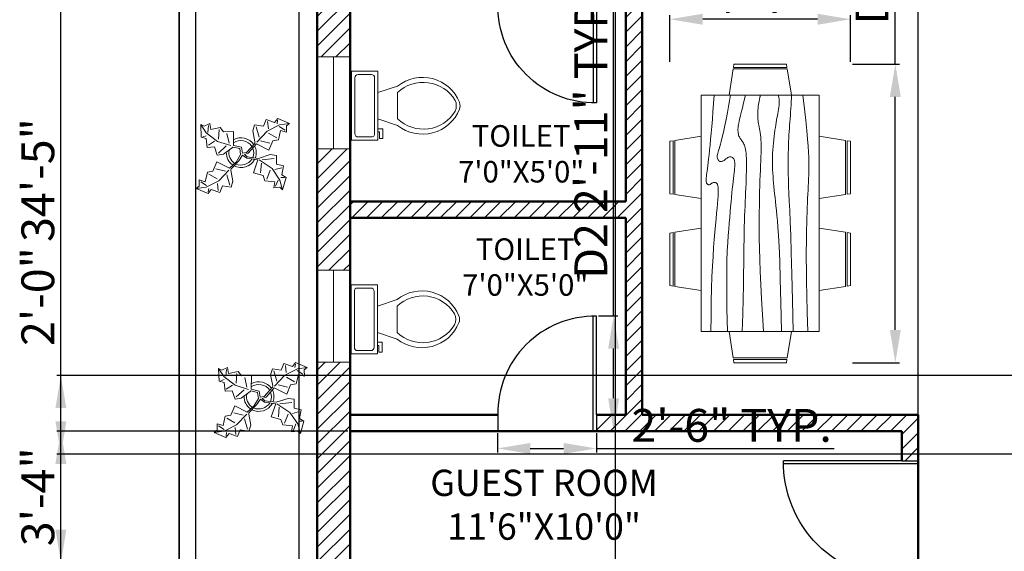
# Model space of a CAD drawing. Units: inches. Extents: x 2206 to 2843, y 1750 to 2489.
# Tile 5 of 8: x 2206 to 2506, y 2075 to 2237. Entities that reach past the tile are written whole.
import ezdxf

# ---------------------------------------------------------------- set-up
doc = ezdxf.new("R2010")
doc.units = ezdxf.units.IN
for name, color, linetype, lineweight in [('A-ANNO-DIMS', 2, 'Continuous', 18), ('A-AREA-IDEN', 7, 'Continuous', 18), ('A-DOOR', 3, 'Continuous', 25), ('A-FLOR-FIXT', 9, 'Continuous', 18), ('A-FURN', 21, 'Continuous', 18), ('A-GLAZ', 4, 'Continuous', 18), ('A-WALL', 7, 'Continuous', 50), ('A-WALL-PATT', 252, 'Continuous', 13), ('C-PROP', 7, 'Continuous', 35), ('L-PLNT', 92, 'Continuous', 18), ('L-SITE-WALL', 8, 'Continuous', 25)]:
    doc.layers.add(name, color=color, linetype=linetype, lineweight=lineweight)
doc.styles.get("Standard").update_dxf_attribs({"font": 'arial.ttf'})
doc.dimstyles.new('ISO-25', dxfattribs={"dimtxt": 10, "dimasz": 10, "dimexe": 1.25, "dimexo": 0.625, "dimtad": 1, "dimdec": 1, "dimlunit": 3, "dimtxsty": 'Standard', "dimcen": 2.5, "dimadec": 0, "dimazin": 0, "dimtfac": 1, "dimtdec": 1, "dimtmove": 0, "dimatfit": 3, "dimfxl": 1, "dimarcsym": 0})

# ---------------------------------------------------------------- blocks, each defined once
blk = doc.blocks.new('Dining Set - 36 x 72 in.')
for p, q in [((-22, 27.5), (-22.1562, 26.50042)), ((-22, 27.5), (-6, 27.5)), ((-5.8437, 26.49966), (-6, 27.5)), ((6, 27.5), (5.8438, 26.50042)), ((6, 27.5), (22, 27.5)), ((22.1563, 26.49966), (22, 27.5)), ((-22.2343, 26.00059), (-23.4847, 17.99762)), ((-22.2304, 26), (-5.7608, 26)), ((-5.8416, 26.5), (-22.1534, 26.5)), ((-4.5152, 17.99762), (-5.7655, 25.99926)), ((5.7657, 26.00059), (4.5153, 17.99762)), ((5.7696, 26), (22.2392, 26)), ((22.1584, 26.5), (5.8466, 26.5)), ((23.4848, 17.99762), (22.2345, 25.99926)), ((36, 18), (-36, 18)), ((-36, 18), (-36, -18)), ((36, -18), (36, 18)), ((-44.0006, 8.23428), (-35.9976, 9.48474)), ((44.0006, 8.23428), (35.9976, 9.48474)), ((-45.5, 8), (-44.5004, 8.15617)), ((-45.5, 8), (-45.5, -8)), ((-44.5, -8.15843), (-44.5, 8.15338)), ((-44, 8.23041), (-44, -8.23915)), ((44, 8.23041), (44, -8.23915)), ((44.5, -8.15843), (44.5, 8.15338)), ((45.5, 8), (44.5005, 8.15617)), ((45.5, 8), (45.5, -8)), ((-44.4997, -8.15631), (-45.5, -8)), ((-35.9976, -9.48476), (-43.9993, -8.2345)), ((35.9976, -9.48476), (43.9993, -8.2345)), ((44.4997, -8.15631), (45.5, -8)), ((-36, -18), (36, -18)), ((-22.2343, -26.0006), (-23.4847, -17.99762)), ((-4.5152, -17.99762), (-5.7655, -25.99928)), ((5.7657, -26.0006), (4.5153, -17.99762)), ((23.4848, -17.99762), (22.2345, -25.99928)), ((-22.2304, -26), (-5.7608, -26)), ((-22, -27.5), (-22.1562, -26.50044)), ((-5.8416, -26.5), (-22.1534, -26.5)), ((-5.8437, -26.49967), (-6, -27.5)), ((5.7696, -26), (22.2392, -26)), ((6, -27.5), (5.8438, -26.50044)), ((22.1584, -26.5), (5.8466, -26.5)), ((22.1563, -26.49967), (22, -27.5)), ((-22, -27.5), (-6, -27.5)), ((6, -27.5), (22, -27.5))]:
    blk.add_line(p, q)
for points in [[(-36, 15), (-31.1772, 14.97754), (-26.8079, 14.91406), (-22.8538, 14.81543), (-19.276, 14.6875), (-16.0362, 14.53613), (-13.0957, 14.36718), (-10.4159, 14.18652), (-7.9583, 14), (-5.6904, 13.81315), (-3.6035, 13.63021), (-1.6954, 13.45508), (0.0365, 13.29166), (1.5945, 13.14388), (2.9811, 13.01562), (4.1988, 12.9108), (5.25, 12.83333), (6.1393, 12.78613), (6.8802, 12.76823), (7.4883, 12.77767), (7.9792, 12.8125), (8.3685, 12.87077), (8.6719, 12.95052), (8.9049, 13.0498), (9.0833, 13.16666), (9.2205, 13.29899), (9.3216, 13.44401), (9.3895, 13.59879), (9.4271, 13.76041), (9.4373, 13.92594), (9.4232, 14.09245), (9.3875, 14.257), (9.3333, 14.41666), (9.2638, 14.56917), (9.1836, 14.71484), (9.0975, 14.85465), (9.0104, 14.98958), (8.9272, 15.1206), (8.8529, 15.2487), (8.7922, 15.37483), (8.75, 15.5), (8.7305, 15.62467), (8.7344, 15.74739), (8.7617, 15.86621), (8.8125, 15.97916), (8.8867, 16.08431), (8.9844, 16.17968), (9.1055, 16.26334), (9.25, 16.33333), (9.4189, 16.38802), (9.6172, 16.42708), (9.8506, 16.45052), (10.125, 16.45833), (10.4463, 16.45052), (10.8203, 16.42708), (11.2529, 16.38802), (11.75, 16.33333), (12.3184, 16.26318), (12.9694, 16.17838), (13.7151, 16.07991), (14.5677, 15.96875), (15.5395, 15.84586), (16.6426, 15.71224), (17.8893, 15.56884), (19.2917, 15.41666), (20.859, 15.25667), (22.5879, 15.08984), (24.4721, 14.91715), (26.5052, 14.73958), (28.6809, 14.5581), (30.9929, 14.3737), (33.4347, 14.18733), (36, 14)], [(-36, 10), (-28.9766, 10.14274), (-23.1725, 10.20442), (-18.4241, 10.19775), (-14.5677, 10.13541), (-11.4399, 10.03011), (-8.877, 9.89453), (-6.7154, 9.74137), (-4.7917, 9.58333), (-2.9698, 9.43082), (-1.2246, 9.28515), (0.4415, 9.14534), (2.026, 9.01041), (3.5266, 8.87939), (4.9408, 8.7513), (6.266, 8.62516), (7.5, 8.5), (8.6411, 8.37549), (9.6914, 8.2539), (10.6538, 8.13818), (11.5312, 8.03125), (12.3267, 7.93603), (13.043, 7.85547), (13.6831, 7.79248), (14.25, 7.75), (14.7471, 7.7303), (15.1797, 7.73307), (15.5537, 7.75732), (15.875, 7.80208), (16.1494, 7.86637), (16.3828, 7.94922), (16.5811, 8.04964), (16.75, 8.16666), (16.8944, 8.29915), (17.0143, 8.44531), (17.1089, 8.60319), (17.1771, 8.77083), (17.218, 8.94629), (17.2305, 9.1276), (17.2137, 9.31282), (17.1667, 9.5), (17.0895, 9.6875), (16.987, 9.875), (16.8649, 10.0625), (16.7292, 10.25), (16.5856, 10.4375), (16.4401, 10.625), (16.2985, 10.8125), (16.1667, 11), (16.05, 11.18733), (15.9518, 11.3737), (15.8752, 11.5581), (15.8229, 11.73958), (15.798, 11.91715), (15.8034, 12.08984), (15.842, 12.25667), (15.9167, 12.41666), (16.0295, 12.56836), (16.1784, 12.70833), (16.3605, 12.83268), (16.5729, 12.9375), (16.8127, 13.01888), (17.0768, 13.07291), (17.3625, 13.0957), (17.6667, 13.08333), (17.9894, 13.03312), (18.3418, 12.94726), (18.7382, 12.82918), (19.1927, 12.68229), (19.7195, 12.51001), (20.3327, 12.31575), (21.0465, 12.10294), (21.875, 11.875), (22.8357, 11.63354), (23.959, 11.37304), (25.2786, 11.08618), (26.8282, 10.76562), (28.6414, 10.40405), (30.752, 9.99414), (33.1936, 9.52856), (36, 9)], [(-36, 5.5), (-30.7157, 5.3348), (-26.069, 5.20963), (-21.9946, 5.11767), (-18.4271, 5.05208), (-15.3009, 5.00602), (-12.5508, 4.97265), (-10.1112, 4.94515), (-7.9167, 4.91666), (-5.909, 4.88167), (-4.0586, 4.83984), (-2.3429, 4.79215), (-0.7396, 4.73958), (0.7739, 4.6831), (2.22, 4.6237), (3.6213, 4.56233), (5, 4.5), (6.373, 4.43782), (7.7344, 4.3776), (9.0723, 4.32129), (10.375, 4.27083), (11.6309, 4.22819), (12.8281, 4.19531), (13.9551, 4.17415), (15, 4.16666), (15.954, 4.17448), (16.819, 4.19791), (17.6001, 4.23698), (18.3021, 4.29166), (18.9299, 4.36198), (19.4883, 4.44791), (19.9823, 4.54948), (20.4167, 4.66666), (20.7969, 4.79899), (21.1302, 4.94401), (21.4245, 5.09879), (21.6875, 5.26041), (21.9271, 5.42594), (22.1511, 5.59245), (22.3672, 5.757), (22.5834, 5.91666), (22.8065, 6.06868), (23.0404, 6.21093), (23.2879, 6.34147), (23.5521, 6.45833), (23.8358, 6.55957), (24.142, 6.64323), (24.4735, 6.70735), (24.8334, 6.75), (25.2235, 6.76969), (25.642, 6.76692), (26.0858, 6.74267), (26.5521, 6.69791), (27.0379, 6.63362), (27.5404, 6.55078), (28.0565, 6.45036), (28.5834, 6.33333), (29.1242, 6.19987), (29.7071, 6.04687), (30.3661, 5.87044), (31.1354, 5.66666), (32.0493, 5.43164), (33.142, 5.16146), (34.4475, 4.85221), (36, 4.5)], [(-36, -1), (-30.7915, -0.6591), (-26.0195, -0.38216), (-21.6519, -0.16284), (-17.6563, 0.00521), (-14.0005, 0.12833), (-10.6523, 0.21289), (-7.5796, 0.26522), (-4.75, 0.29166), (-2.134, 0.29793), (0.2878, 0.28711), (2.5317, 0.26163), (4.6146, 0.22396), (6.5529, 0.17651), (8.3633, 0.12174), (10.0623, 0.06209), (11.6667, 0), (13.1899, -0.06201), (14.6341, -0.1211), (15.9982, -0.17432), (17.2813, -0.21875), (18.4823, -0.25147), (19.6003, -0.26953), (20.6343, -0.27002), (21.5834, -0.25), (22.4481, -0.20768), (23.2357, -0.14584), (23.9549, -0.06836), (24.6146, 0.02083), (25.2235, 0.11784), (25.7904, 0.21875), (26.3241, 0.31966), (26.8334, 0.41666), (27.3265, 0.50618), (27.8099, 0.58593), (28.2894, 0.65397), (28.7709, 0.70833), (29.2601, 0.74707), (29.763, 0.76823), (30.2855, 0.76985), (30.8334, 0.75), (31.4088, 0.70784), (31.9994, 0.64713), (32.589, 0.57275), (33.1615, 0.48958), (33.7008, 0.4025), (34.1908, 0.3164), (34.6153, 0.23616), (34.9584, 0.16666), (35.2099, 0.11165), (35.3848, 0.07031), (35.504, 0.04069), (35.5886, 0.02083), (35.6594, 0.00879), (35.7377, 0.0026), (35.8442, 0.00032), (36, 0)], [(-36, -6.5), (-27.1843, -6.31267), (-20.084, -6.1263), (-14.469, -5.9419), (-10.1094, -5.76042), (-6.7752, -5.58285), (-4.2363, -5.41016), (-2.2629, -5.24333), (-0.625, -5.08334), (0.8708, -4.93099), (2.2715, -4.78646), (3.5872, -4.64974), (4.8281, -4.52084), (6.0046, -4.39974), (7.127, -4.28646), (8.2053, -4.18099), (9.25, -4.08334), (10.2705, -3.99382), (11.2734, -3.91407), (12.2647, -3.84603), (13.25, -3.79167), (14.2354, -3.75293), (15.2266, -3.73177), (16.2295, -3.73015), (17.25, -3.75), (18.2912, -3.79248), (19.3451, -3.85547), (20.4009, -3.93604), (21.4479, -4.03125), (22.4754, -4.13819), (23.4727, -4.25391), (24.4289, -4.37549), (25.3334, -4.5), (26.1785, -4.62492), (26.9694, -4.74935), (27.7145, -4.87281), (28.4219, -4.99479), (29.1, -5.11483), (29.7572, -5.23242), (30.4016, -5.34709), (31.0417, -5.45834), (31.6837, -5.56437), (32.3262, -5.65821), (32.9658, -5.73153), (33.599, -5.77604), (34.2224, -5.78345), (34.8327, -5.74545), (35.4264, -5.65373), (36, -5.5)], [(-36, -10), (-26.4022, -9.81299), (-18.4675, -9.62891), (-11.9839, -9.45069), (-6.7396, -9.28125), (-2.5226, -9.12354), (0.8789, -8.98047), (3.6769, -8.85498), (6.0833, -8.75), (8.2767, -8.66765), (10.3021, -8.60677), (12.1712, -8.56543), (13.8958, -8.54167), (15.4876, -8.53353), (16.9583, -8.53907), (18.3197, -8.55632), (19.5834, -8.58334), (20.7616, -8.61841), (21.8685, -8.66081), (22.9188, -8.71004), (23.9271, -8.76563), (24.9081, -8.82707), (25.8763, -8.89388), (26.8465, -8.96558), (27.8334, -9.04167), (28.8474, -9.12118), (29.8828, -9.20117), (30.93, -9.27824), (31.9792, -9.34896), (33.0205, -9.40991), (34.0443, -9.45768), (35.0407, -9.48885), (36, -9.5)], [(-36, -14.5), (-30.0881, -14.33513), (-25.0332, -14.21224), (-20.7312, -14.12647), (-17.0781, -14.07292), (-13.97, -14.04671), (-11.3027, -14.04297), (-8.9724, -14.05681), (-6.875, -14.08334), (-4.9224, -14.11833), (-3.0905, -14.16016), (-1.3709, -14.20785), (0.2448, -14.26042), (1.7647, -14.3169), (3.1973, -14.3763), (4.5507, -14.43767), (5.8333, -14.5), (7.0554, -14.5621), (8.235, -14.62175), (9.3922, -14.67652), (10.5469, -14.72396), (11.7192, -14.76164), (12.929, -14.78711), (14.1965, -14.79794), (15.5417, -14.79167), (16.9933, -14.76424), (18.6152, -14.70508), (20.4804, -14.60197), (22.6615, -14.44271), (25.2312, -14.21509), (28.2624, -13.9069), (31.8277, -13.50594), (36, -13)]]:
    blk.add_lwpolyline(points)
blk = doc.blocks.new('Toilet - top')
for p, q in [((9.5, -6), (9.5, -2)), ((-10, -8.5), (-8, -8.5)), ((-10, -9.5), (-10, -8.5)), ((-8, -8.5), (-8, -8)), ((-7, -8), (-7, -9.5)), ((-4, -8), (-6, -14)), ((4, -8), (6, -14)), ((-7, -9.5), (-10, -9.5)), ((4, -14), (-4, -14))]:
    blk.add_line(p, q)
blk.add_lwpolyline([(10.5, -8), (10.5, 0), (-10.5, 0), (-10.5, -8)], close=True)
for points in [[(-9.5, -2), (-9.5, -6)], [(8.5, -1), (-8.5, -1)], [(-8.5, -7), (8.5, -7)]]:
    blk.add_lwpolyline(points)
for centre, radius, start, end in [((-8.62, -1.88), 0.884, 81.8699, 188.1301), ((8.62, -1.88), 0.884, 351.8699, 98.1301), ((-8.62, -6.12), 0.884, 171.8699, 278.1301), ((8.62, -6.12), 0.884, 261.8699, 8.1301), ((3.52, -21.58), 12.17, 141.4691, 247.9714), ((4.2, -21.82), 11.33, 136.3677, 238.9468), ((-3.52, -21.58), 12.17, 292.0284, 38.5307), ((-4.2, -21.82), 11.33, 301.053, 43.6321), ((0, -27.88), 4, 245.7318, 294.2682), ((0, -29), 4, 254.8605, 285.1395)]:
    blk.add_arc(centre, radius, start, end)
blk = doc.blocks.new('Plant - Rubber or Philodendron')
for p, q in [((-14.8639, 10.7964), (-12.6195, 11.8975)), ((-12.6195, 11.8975), (-12.1909, 9.4345)), ((8.8871, 10.7908), (9.9809, 13.4933)), ((9.9809, 13.4933), (13.3837, 12.301)), ((10.5828, 12.6946), (10.8893, 9.7953)), ((13.3837, 12.301), (14.68, 13.9039)), ((14.5816, 13.2037), (14.3848, 11.8033)), ((14.68, 13.9039), (19.3848, 11.8146)), ((-16.2005, 11.4774), (-13.9899, 8.1064)), ((-16.2005, 11.4774), (-14.8639, 10.7964)), ((-16.0159, 6.3329), (-16.2005, 11.4774)), ((-13.9899, 8.1064), (-9.5434, 4.7185)), ((-13.3174, 8.325), (-13.0735, 11.0065)), ((-12.1909, 9.4345), (-8.3829, 10.3)), ((-8.8369, 9.409), (-9.0894, 5.6095)), ((-8.3829, 10.3), (-7.0549, 8.501)), ((-7.0549, 8.501), (-3.0284, 8.6941)), ((-3.0284, 8.6941), (-3.0709, 3.1041)), ((4.6914, 8.8812), (5.3859, 11.2828)), ((4.6914, 8.8812), (5.5014, 4.4831)), ((5.3859, 11.2828), (8.8871, 10.7908)), ((5.9878, 10.4842), (7.1971, 6.3869)), ((10.3916, 8.7942), (6.2847, 4.4028)), ((15.3859, 11.3055), (10.3916, 8.7942)), ((14.2977, 6.1031), (10.9934, 7.9956)), ((15.7909, 9.1065), (14.8995, 5.3044)), ((15.2875, 10.6053), (17.5907, 9.2105)), ((19.3848, 11.8146), (15.3859, 11.3055)), ((18.1925, 8.4119), (15.7909, 9.1065)), ((19.3848, 11.8146), (18.1868, 10.9119)), ((18.1868, 10.9119), (18.1925, 8.4119)), ((-14.0069, 5.8704), (-16.0159, 6.3329)), ((-15.3434, 6.5514), (-13.9984, 6.9884)), ((-13.5868, 2.2894), (-14.0069, 5.8704)), ((-13.1329, 3.1804), (-10.6614, 4.727)), ((-9.5434, 4.7185), (-4.1917, 2.9888)), ((-4.8529, 4.012), (-5.7184, 7.82)), ((5.4346, 3.9146), (5.5014, 4.4831)), ((7.7005, 4.8881), (11.5025, 3.9967)), ((12.7005, 4.8994), (11.1089, 1.1958)), ((14.8995, 5.3044), (12.7005, 4.8994)), ((-10.6784, 2.491), (-13.5868, 2.2894)), ((-9.5858, -0.8715), (-10.6784, 2.491)), ((-9.1318, 0.0195), (-5.9793, 2.9025)), ((-7.1228, -0.443), (-3.5248, 2.2131)), ((-3.5248, 2.2131), (-3.3011, 2.4355)), ((-3.3011, 2.4355), (-0.5306, 1.7947)), ((-3.0709, 3.1041), (0.0797, 2.3163)), ((-0.5306, 1.7947), (-0.2255, -0.5527)), ((-0.5306, 1.7947), (-0.5306, 1.7947)), ((0.0797, 2.3163), (0.4866, -0.031)), ((0.4866, -0.031), (2.1141, 0.2298)), ((2.1141, 0.2298), (5.4346, 3.9146)), ((6.1032, 3.6844), (2.8262, -0.031)), ((11.1089, 1.1958), (6.1032, 3.6844)), ((-11.3237, -7.2629), (-9.7321, -3.5593)), ((-9.7321, -3.5593), (-4.7264, -6.0479)), ((-7.1228, -0.443), (-9.5858, -0.8715)), ((-2.019, -3.6148), (-4.7264, -6.0479)), ((-4.0579, -6.2781), (-0.9375, -3.1608)), ((-2.019, -3.6148), (-0.2255, -0.5527)), ((-0.9375, -3.1608), (0.5883, -0.8135)), ((0.5883, -0.8135), (2.2447, -2.0916)), ((2.8262, -0.031), (1.3003, -0.5527)), ((1.3003, -0.5527), (2.4193, -1.4655)), ((2.2447, -2.0916), (6.7108, -2.6626)), ((2.4193, -1.4655), (6.895, -2.1175)), ((4.943, -7.9659), (6.7108, -2.6626)), ((11.6605, -0.5413), (6.895, -2.1175)), ((12.3677, -6.1981), (7.219, -2.6772)), ((8.3544, -2.7453), (13.1973, -2.1704)), ((11.6605, -0.5413), (14.1354, -0.8948)), ((14.1354, -0.8948), (14.1354, -4.4304)), ((-14.4141, -11.4699), (-13.5228, -7.6679)), ((-13.5228, -7.6679), (-11.3237, -7.2629)), ((-6.3237, -7.2516), (-10.1257, -6.3602)), ((-9.0148, -11.1577), (-4.9047, -6.8122)), ((-4.1246, -6.8466), (-4.0579, -6.2781)), ((-3.3146, -11.2447), (-4.1246, -6.8466)), ((8.125, -4.0768), (7.7715, -7.9659)), ((10.2463, -10.4408), (11.6605, -6.9053)), ((15.5496, -10.7943), (12.3677, -6.1981)), ((16.2567, -5.8446), (13.4283, -6.5517)), ((14.1354, -4.4304), (16.9638, -5.1375)), ((16.9638, -5.1375), (16.2567, -8.673)), ((-16.8157, -10.7754), (-14.4141, -11.4699)), ((-16.8101, -13.2754), (-16.8157, -10.7754)), ((-13.9107, -12.9688), (-16.2139, -11.574)), ((-14.0091, -13.669), (-9.0148, -11.1577)), ((-12.921, -8.4665), (-9.6166, -10.359)), ((-4.611, -12.8477), (-5.8203, -8.7504)), ((-3.3146, -11.2447), (-4.0092, -13.6463)), ((8.8321, -9.0266), (4.943, -7.9659)), ((9.5392, -11.1479), (8.8321, -9.0266)), ((13.4283, -11.5015), (9.5392, -11.1479)), ((13.0748, -13.9763), (13.4283, -11.5015)), ((14.8425, -10.7943), (13.7819, -13.2692)), ((16.6103, -14.6834), (15.5496, -10.7943)), ((17.3174, -9.7337), (15.9032, -9.7337)), ((16.2567, -8.673), (18.0245, -9.7337)), ((18.0245, -9.7337), (16.6103, -14.6834)), ((-18.008, -14.1781), (-16.8101, -13.2754)), ((-18.008, -14.1781), (-14.0091, -13.669)), ((-13.3032, -16.2674), (-18.008, -14.1781)), ((-12.0069, -14.6645), (-13.3032, -16.2674)), ((-13.2048, -15.5672), (-13.008, -14.1668)), ((-8.6042, -15.8568), (-12.0069, -14.6645)), ((-9.206, -15.0581), (-9.5126, -12.1588)), ((-7.5103, -13.1543), (-8.6042, -15.8568)), ((-4.0092, -13.6463), (-7.5103, -13.1543)), ((15.5496, -13.6228), (13.0748, -13.9763)), ((16.6103, -14.6834), (15.5496, -13.6228))]:
    blk.add_line(p, q)
for centre, radius, start, end in [((0, 0), 6.1275, 34.37569, 120.1028), ((-0.0601, -0.2075), 5.2461, 33.82192, 124.9414), ((0.0308, 0.1664), 6, 178.6147, 235.1169), ((0.0308, 0.1664), 5, 168.1647, 238.6725), ((-0.2664, 0.1682), 5.2775, 338.4094, 20.03007), ((-0.098, 0.1364), 6.1288, 341.2017, 26.09184), ((-0.0234, 0.3825), 6.1492, 242.5812, 331.2714), ((-0.1102, 0.4886), 5.2883, 247.3711, 327.472)]:
    blk.add_arc(centre, radius, start, end)
blk = doc.blocks.new('WIN-28IN')
for p, q in [((10, 28), (0, 28)), ((5, 28), (5, 0)), ((10, 0), (0, 0))]:
    blk.add_line(p, q)
blk = doc.blocks.new('DOOR-SWING-36IN')
for p, q in [((0, 5), (0, 41)), ((1, 0), (1, 41)), ((0, 5), (0, 0)), ((36, 5), (36, 0))]:
    blk.add_line(p, q)
blk.add_arc((0.5, 5.5), 35.5, 359.1931, 90.8069)
blk = doc.blocks.new('DOOR-SWING-30IN')
for p, q in [((29, 0), (29, 35)), ((30, 5), (30, 35))]:
    blk.add_line(p, q)
blk.add_arc((29.5, 5.5), 29.5, 89.029, 180.971)
blk = doc.blocks.new('*D43')
at = {"layer": 'A-ANNO-DIMS', "color": 0, "lineweight": -2, "transparency": 16777216}
for p, q in [((2386.85, 2147.03), (2386.85, 2248.25)), ((2382.2, 2147.03), (2388.1, 2147.03)), ((2386.85, 2121.9), (2386.85, 2137.03)), ((2382.2, 2111.9), (2388.1, 2111.9))]:
    blk.add_line(p, q, dxfattribs=at)
at = {"layer": 'A-ANNO-DIMS', "color": 0, "transparency": 16777216}
for points in [[(2385.18, 2137.03), (2388.52, 2137.03), (2386.85, 2147.03)], [(2385.18, 2121.9), (2388.52, 2121.9), (2386.85, 2111.9)]]:
    blk.add_solid(points, dxfattribs=at)
at = {"layer": 'Defpoints', "color": 0, "transparency": 16777216}
for p in [(2381.58, 2147.03), (2386.85, 2147.03), (2381.58, 2111.9)]:
    blk.add_point(p, dxfattribs=at)
at = {"layer": 'A-ANNO-DIMS', "color": 0, "transparency": 16777216, "insert": (2381.2, 2202.64), "char_height": 10, "attachment_point": 5, "rotation": 90}
blk.add_mtext('D2 2\'-11" TYP.', dxfattribs=at)
blk = doc.blocks.new('*D44')
at = {"layer": 'A-ANNO-DIMS', "color": 0, "lineweight": -2, "transparency": 16777216}
for p, q in [((2351.44, 2111.27), (2351.44, 2105.38)), ((2381.58, 2111.27), (2381.58, 2105.38)), ((2361.44, 2106.63), (2371.58, 2106.63)), ((2381.58, 2106.63), (2453.96, 2106.63))]:
    blk.add_line(p, q, dxfattribs=at)
at = {"layer": 'A-ANNO-DIMS', "color": 0, "transparency": 16777216}
for points in [[(2361.44, 2108.3), (2361.44, 2104.96), (2351.44, 2106.63)], [(2371.58, 2108.3), (2371.58, 2104.96), (2381.58, 2106.63)]]:
    blk.add_solid(points, dxfattribs=at)
at = {"layer": 'Defpoints', "color": 0, "transparency": 16777216}
for p in [(2351.44, 2111.9), (2381.58, 2111.9), (2381.58, 2106.63)]:
    blk.add_point(p, dxfattribs=at)
at = {"layer": 'A-ANNO-DIMS', "color": 0, "transparency": 16777216, "insert": (2422.77, 2112.36), "char_height": 10, "attachment_point": 5}
blk.add_mtext('2\'-6" TYP.', dxfattribs=at)
blk = doc.blocks.new('*D47')
at = {"layer": 'A-ANNO-DIMS', "color": 0, "lineweight": -2, "transparency": 16777216}
for p, q in [((2472.62, 2223.74), (2472.62, 2344.9)), ((2459.59, 2223.74), (2473.87, 2223.74)), ((2472.62, 2142.74), (2472.62, 2213.74)), ((2459.59, 2132.74), (2473.87, 2132.74))]:
    blk.add_line(p, q, dxfattribs=at)
at = {"layer": 'A-ANNO-DIMS', "color": 0, "transparency": 16777216}
for points in [[(2470.95, 2213.74), (2474.28, 2213.74), (2472.62, 2223.74)], [(2470.95, 2142.74), (2474.28, 2142.74), (2472.62, 2132.74)]]:
    blk.add_solid(points, dxfattribs=at)
at = {"layer": 'Defpoints', "color": 0, "transparency": 16777216}
for p in [(2458.97, 2223.74), (2472.62, 2223.74), (2458.97, 2132.74)]:
    blk.add_point(p, dxfattribs=at)
at = {"layer": 'A-ANNO-DIMS', "color": 0, "transparency": 16777216, "insert": (2466.82, 2289.32), "char_height": 10, "attachment_point": 5, "rotation": 90}
blk.add_mtext('DINING SET 7\'-7"', dxfattribs=at)
blk = doc.blocks.new('*D48')
at = {"layer": 'A-ANNO-DIMS', "color": 0, "lineweight": -2, "transparency": 16777216}
for p, q in [((2403.97, 2224.37), (2403.97, 2238.64)), ((2448.97, 2237.39), (2413.97, 2237.39)), ((2458.97, 2224.37), (2458.97, 2238.64))]:
    blk.add_line(p, q, dxfattribs=at)
at = {"layer": 'A-ANNO-DIMS', "color": 0, "transparency": 16777216}
for points in [[(2413.97, 2239.06), (2413.97, 2235.73), (2403.97, 2237.39)], [(2448.97, 2239.06), (2448.97, 2235.73), (2458.97, 2237.39)]]:
    blk.add_solid(points, dxfattribs=at)
at = {"layer": 'Defpoints', "color": 0, "transparency": 16777216}
for p in [(2403.97, 2237.39), (2403.97, 2223.74), (2458.97, 2223.74)]:
    blk.add_point(p, dxfattribs=at)
at = {"layer": 'A-ANNO-DIMS', "color": 0, "transparency": 16777216, "insert": (2431.47, 2243.02), "char_height": 10, "attachment_point": 5}
blk.add_mtext('4\'-7"', dxfattribs=at)
blk = doc.blocks.new('*D58')
at = {"layer": 'A-ANNO-DIMS', "color": 0, "lineweight": -2, "transparency": 16777216}
for p, q in [((2295.95, 2394.9), (2217.28, 2394.9)), ((2218.53, 1991.9), (2218.53, 2384.9)), ((2295.95, 1981.9), (2217.28, 1981.9))]:
    blk.add_line(p, q, dxfattribs=at)
at = {"layer": 'A-ANNO-DIMS', "color": 0, "transparency": 16777216}
for points in [[(2216.86, 2384.9), (2220.2, 2384.9), (2218.53, 2394.9)], [(2216.86, 1991.9), (2220.2, 1991.9), (2218.53, 1981.9)]]:
    blk.add_solid(points, dxfattribs=at)
at = {"layer": 'Defpoints', "color": 0, "transparency": 16777216}
for p in [(2218.53, 2394.9), (2296.58, 2394.9), (2296.58, 1981.9)]:
    blk.add_point(p, dxfattribs=at)
at = {"layer": 'A-ANNO-DIMS', "color": 0, "transparency": 16777216, "insert": (2212.8, 2188.4), "char_height": 10, "attachment_point": 5, "rotation": 90}
blk.add_mtext('34\'-5"', dxfattribs=at)
blk = doc.blocks.new('*D61')
at = {"layer": 'A-ANNO-DIMS', "color": 0, "lineweight": -2, "transparency": 16777216}
for p, q in [((2479.58, 2100.52), (2479.58, 2432.2)), ((2521.58, 2100.52), (2521.58, 2432.2)), ((2489.58, 2430.95), (2511.58, 2430.95))]:
    blk.add_line(p, q, dxfattribs=at)
at = {"layer": 'A-ANNO-DIMS', "color": 0, "transparency": 16777216}
for points in [[(2489.58, 2432.62), (2489.58, 2429.28), (2479.58, 2430.95)], [(2511.58, 2432.62), (2511.58, 2429.28), (2521.58, 2430.95)]]:
    blk.add_solid(points, dxfattribs=at)
at = {"layer": 'Defpoints', "color": 0, "transparency": 16777216}
for p in [(2521.58, 2430.95), (2479.58, 2099.9), (2521.58, 2099.9)]:
    blk.add_point(p, dxfattribs=at)
at = {"layer": 'A-ANNO-DIMS', "color": 0, "transparency": 16777216, "insert": (2500.58, 2436.68), "char_height": 10, "attachment_point": 5}
blk.add_mtext('3\'-6"', dxfattribs=at)
blk = doc.blocks.new('*D67')
at = {"layer": 'A-ANNO-DIMS', "color": 0, "lineweight": -2, "transparency": 16777216}
for p, q in [((2305.95, 2111.9), (2217.28, 2111.9)), ((2218.53, 2081.9), (2218.53, 2101.9)), ((2305.95, 2071.9), (2217.28, 2071.9))]:
    blk.add_line(p, q, dxfattribs=at)
at = {"layer": 'A-ANNO-DIMS', "color": 0, "transparency": 16777216}
for points in [[(2216.86, 2101.9), (2220.2, 2101.9), (2218.53, 2111.9)], [(2216.86, 2081.9), (2220.2, 2081.9), (2218.53, 2071.9)]]:
    blk.add_solid(points, dxfattribs=at)
at = {"layer": 'Defpoints', "color": 0, "transparency": 16777216}
for p in [(2218.53, 2111.9), (2306.58, 2111.9), (2306.58, 2071.9)]:
    blk.add_point(p, dxfattribs=at)
at = {"layer": 'A-ANNO-DIMS', "color": 0, "transparency": 16777216, "insert": (2212.8, 2091.9), "char_height": 10, "attachment_point": 5, "rotation": 90}
blk.add_mtext('3\'-4"', dxfattribs=at)
blk = doc.blocks.new('*D72')
at = {"layer": 'A-ANNO-DIMS', "color": 0, "lineweight": -2, "transparency": 16777216}
for p, q in [((2291.11, 1795.52), (2291.11, 2432.2)), ((2387.37, 1795.52), (2387.37, 2432.2)), ((2301.11, 2430.95), (2377.37, 2430.95))]:
    blk.add_line(p, q, dxfattribs=at)
at = {"layer": 'A-ANNO-DIMS', "color": 0, "transparency": 16777216}
for points in [[(2301.11, 2432.62), (2301.11, 2429.28), (2291.11, 2430.95)], [(2377.37, 2432.62), (2377.37, 2429.28), (2387.37, 2430.95)]]:
    blk.add_solid(points, dxfattribs=at)
at = {"layer": 'Defpoints', "color": 0, "transparency": 16777216}
for p in [(2387.37, 2430.95), (2291.11, 1794.9), (2387.37, 1794.9)]:
    blk.add_point(p, dxfattribs=at)
at = {"layer": 'A-ANNO-DIMS', "color": 0, "transparency": 16777216, "insert": (2339.24, 2436.74), "char_height": 10, "attachment_point": 5}
blk.add_mtext('8\'-0 1/2"', dxfattribs=at)
blk = doc.blocks.new('*D78')
at = {"layer": 'A-ANNO-DIMS', "color": 0, "lineweight": -2, "transparency": 16777216}
for p, q in [((2218.53, 2128.9), (2218.53, 2166.9)), ((2545.59, 2128.9), (2217.28, 2128.9)), ((2218.53, 2114.9), (2218.53, 2118.9)), ((2545.59, 2104.9), (2217.28, 2104.9))]:
    blk.add_line(p, q, dxfattribs=at)
at = {"layer": 'A-ANNO-DIMS', "color": 0, "transparency": 16777216}
for points in [[(2216.86, 2118.9), (2220.2, 2118.9), (2218.53, 2128.9)], [(2216.86, 2114.9), (2220.2, 2114.9), (2218.53, 2104.9)]]:
    blk.add_solid(points, dxfattribs=at)
at = {"layer": 'Defpoints', "color": 0, "transparency": 16777216}
for p in [(2218.53, 2128.9), (2546.21, 2128.9), (2546.21, 2104.9)]:
    blk.add_point(p, dxfattribs=at)
at = {"layer": 'A-ANNO-DIMS', "color": 0, "transparency": 16777216, "insert": (2212.8, 2152.9), "char_height": 10, "attachment_point": 5, "rotation": 90}
blk.add_mtext('2\'-0"', dxfattribs=at)

msp = doc.modelspace()

# ---------------------------------------------------------------- hatches: boundary and pattern name
at = {"layer": 'A-WALL-PATT'}
h = msp.add_hatch(dxfattribs=at)
h.set_pattern_fill('ANSI31', color=256)
h.paths.add_polyline_path([(2710.58, 2394.9), (2296.58, 2394.9), (2296.58, 2335.9), (2306.58, 2335.9), (2306.58, 2384.9), (2479.58, 2384.9), (2652.58, 2384.9), (2700.58, 2384.9), (2700.58, 2300.9), (2690.58, 2300.9), (2690.58, 2290.9), (2710.58, 2290.9)])
h.paths.add_polyline_path([(2306.58, 2295.9), (2296.58, 2295.9), (2296.58, 2225.9), (2306.58, 2225.9), (2306.58, 2241.9)])
h.paths.add_polyline_path([(2306.58, 2111.9), (2306.58, 2132.9), (2296.58, 2132.9), (2296.58, 2071.9), (2306.58, 2071.9)])
h.paths.add_polyline_path([(2306.58, 2197.9), (2296.58, 2197.9), (2296.58, 2160.9), (2306.58, 2160.9), (2306.58, 2176.9)])
h.paths.add_polyline_path([(2370.58, 1991.9), (2306.58, 1991.9), (2306.58, 2031.9), (2296.58, 2031.9), (2296.58, 1981.9), (2370.58, 1981.9)])
h.paths.add_polyline_path([(2479.58, 2066.9), (2474.58, 2066.9), (2474.58, 1991.9), (2410.58, 1991.9), (2410.58, 1981.9), (2479.58, 1981.9)])
h.paths.add_polyline_path([(2539.58, 1943.9), (2479.58, 1943.9), (2479.58, 1944.9), (2469.58, 1944.9), (2469.58, 1933.9), (2539.58, 1933.9)])
h.paths.add_polyline_path([(2657.58, 1997.9), (2647.58, 1997.9), (2647.58, 1943.9), (2647.58, 1918.9), (2657.58, 1918.9)])
h.paths.add_polyline_path([(2647.58, 1943.9), (2587.58, 1943.9), (2587.58, 1933.9), (2647.58, 1933.9)])
h.paths.add_polyline_path([(2657.58, 2158.4), (2647.58, 2158.4), (2647.58, 2104.9), (2647.58, 2045.9), (2657.58, 2045.9)])
h.paths.add_polyline_path([(2657.58, 2204.89), (2647.58, 2204.89), (2647.58, 2188.4), (2657.58, 2188.4)])
h.paths.add_polyline_path([(2657.58, 2246.9), (2647.58, 2246.9), (2647.58, 2234.9), (2657.58, 2234.9)])
h.paths.add_polyline_path([(2662.58, 2300.9), (2652.58, 2300.9), (2652.58, 2346.22), (2647.58, 2346.22), (2647.58, 2290.9), (2662.58, 2290.9)])
h.paths.add_polyline_path([(2647.58, 2246.9), (2524.58, 2246.9), (2524.58, 2241.9), (2647.58, 2241.9)])
h.paths.add_polyline_path([(2351.58, 2246.9), (2306.58, 2246.9), (2306.58, 2241.9), (2351.58, 2241.9)])
h.paths.add_polyline_path([(2429.58, 2246.9), (2381.58, 2246.9), (2381.58, 2241.9), (2390.58, 2241.9), (2390.58, 2181.9), (2306.58, 2181.9), (2306.58, 2176.9), (2390.58, 2176.9), (2390.58, 2116.9), (2381.58, 2116.9), (2381.58, 2111.9), (2474.58, 2111.9), (2474.58, 2102.9), (2479.58, 2102.9), (2479.58, 2104.9), (2479.58, 2116.9), (2395.58, 2116.9), (2395.58, 2176.9), (2395.58, 2241.9), (2429.58, 2241.9)])
h.paths.add_polyline_path([(2479.58, 2384.9), (2474.58, 2384.9), (2474.58, 2246.9), (2465.58, 2246.9), (2465.58, 2241.9), (2479.58, 2241.9), (2488.58, 2241.9), (2488.58, 2246.9), (2479.58, 2246.9)])
h.paths.add_polyline_path([(2657.58, 1870.9), (2647.58, 1870.9), (2647.58, 1855.9), (2511.58, 1855.9), (2511.58, 1845.9), (2657.58, 1845.9)])

# ---------------------------------------------------------------- linework, layer by layer
at = {"layer": 'A-DOOR'}
for p, q in [((2351.58, 2116.9), (2351.58, 2111.9)), ((2381.58, 2116.9), (2381.58, 2111.9))]:
    msp.add_line(p, q, dxfattribs=at)
at = {"layer": 'A-WALL'}
for p, q in [((2296.58, 1981.9), (2296.58, 2394.9)), ((2306.58, 2176.9), (2306.58, 2241.9)), ((2390.58, 2181.9), (2390.58, 2241.9)), ((2395.58, 2176.9), (2395.58, 2241.9)), ((2306.58, 2181.9), (2390.58, 2181.9)), ((2306.58, 2176.9), (2390.58, 2176.9)), ((2306.58, 2111.9), (2306.58, 2176.9)), ((2390.58, 2116.9), (2390.58, 2176.9)), ((2395.58, 2116.9), (2395.58, 2176.9)), ((2306.58, 2116.9), (2351.58, 2116.9)), ((2381.58, 2116.9), (2390.58, 2116.9)), ((2395.58, 2116.9), (2479.58, 2116.9)), ((2479.58, 2116.9), (2479.58, 2104.9)), ((2306.58, 2111.9), (2474.58, 2111.9)), ((2306.58, 1991.9), (2306.58, 2111.9)), ((2474.58, 2102.9), (2474.58, 2111.9)), ((2479.58, 2104.9), (2479.58, 2099.9)), ((2479.58, 2099.9), (2479.58, 1981.9))]:
    msp.add_line(p, q, dxfattribs=at)
at = {"layer": 'C-PROP'}
msp.add_line((2254.58, 1794.9), (2254.58, 2394.9), dxfattribs=at)
at = {"layer": 'L-SITE-WALL'}
msp.add_line((2259.58, 1799.9), (2259.58, 2384.9), dxfattribs=at)

# ---------------------------------------------------------------- block references
at = {"layer": 'A-DOOR', "extrusion": (0, 0, -1), "zscale": -1}
for name, p, rotation in [('DOOR-SWING-30IN', (-2351.58, 2246.9), 180), ('DOOR-SWING-36IN', (-2479.58, 2102.9), 270.0000000000001)]:
    msp.add_blockref(name, p, dxfattribs=dict(at, rotation=rotation))
at = {"layer": 'A-DOOR'}
msp.add_blockref('DOOR-SWING-30IN', (2351.58, 2111.9), dxfattribs=at)
at = {"layer": 'A-FLOR-FIXT', "rotation": 90}
for p in [(2307.06, 2211.04), (2306.89, 2145.97)]:
    msp.add_blockref('Toilet - top', p, dxfattribs=at)
at = {"layer": 'A-FURN', "rotation": 90}
msp.add_blockref('Dining Set - 36 x 72 in.', (2431.47, 2178.24), dxfattribs=at)
at = {"layer": 'A-GLAZ'}
msp.add_blockref('WIN-28IN', (2296.58, 2197.9), dxfattribs=at)
at = {"layer": 'A-GLAZ', "rotation": 180}
msp.add_blockref('WIN-28IN', (2306.58, 2160.9), dxfattribs=at)
at = {"layer": 'L-PLNT', "xscale": 0.7595985084536371, "yscale": 0.7595985084536371, "zscale": 0.7595985084536371}
for p in [(2273.43, 2196.61), (2278.84, 2122.29)]:
    msp.add_blockref('Plant - Rubber or Philodendron', p, dxfattribs=at)

# ---------------------------------------------------------------- texts
at = {"layer": 'A-AREA-IDEN', "attachment_point": 1}
for s, width, gutter_width, insert, char_height in [('\\pxqc;TOILET\\P7\'0"X5\'0"', 75.366, 10.24, (2321, 2205.13), 6.5536), ('\\pxqc;TOILET\\P7\'0"X5\'0"', 75.366, 10.24, (2322.23, 2170.63), 6.5536), ('\\pxqc;GUEST ROOM\\P11\'6"X10\'0"', 91.9993, 12.5, (2319.64, 2100.15), 8)]:
    msp.add_mtext_dynamic_manual_height_columns(s, width=width, gutter_width=gutter_width, heights=[0], dxfattribs=dict(at, insert=insert, char_height=char_height))

# ---------------------------------------------------------------- dimensions: what is measured, and where the dimension line sits
at = {"layer": 'A-ANNO-DIMS'}
for base, p1, p2, picture, middle in [((2387.37, 2430.95), (2291.11, 1794.9), (2387.37, 1794.9), '*D72', (2339.24, 2436.74)), ((2521.58, 2430.95), (2479.58, 2099.9), (2521.58, 2099.9), '*D61', (2500.58, 2436.68))]:
    dim = msp.add_linear_dim(base=base, p1=p1, p2=p2, dimstyle='ISO-25', override={"dimdec": 1, "dimlfac": 1, "dimrnd": 0, "dimzin": 1, "dimdsep": 46, "dimlunit": 4, "dimfrac": 2}, dxfattribs=at)
    dim.commit()
    dim.dimension.update_dxf_attribs({"geometry": picture, "text_midpoint": middle})
for base, p1, p2, angle, picture, middle in [((2218.53, 2394.9), (2296.58, 1981.9), (2296.58, 2394.9), 90, '*D58', (2212.8, 2188.4)), ((2403.97, 2237.39), (2458.97, 2223.74), (2403.97, 2223.74), 180, '*D48', (2431.47, 2243.02)), ((2218.53, 2128.9), (2546.21, 2104.9), (2546.21, 2128.9), 90, '*D78', (2212.8, 2152.9)), ((2218.53, 2111.9), (2306.58, 2071.9), (2306.58, 2111.9), 90, '*D67', (2212.8, 2091.9))]:
    dim = msp.add_linear_dim(base=base, p1=p1, p2=p2, angle=angle, dimstyle='ISO-25', override={"dimdec": 1, "dimlfac": 1, "dimrnd": 0, "dimzin": 1, "dimdsep": 46, "dimlunit": 4, "dimfrac": 2}, dxfattribs=at)
    dim.commit()
    dim.dimension.update_dxf_attribs({"geometry": picture, "text_midpoint": middle})
for base, p1, p2, text, picture, middle in [((2472.62, 2223.74), (2458.97, 2132.74), (2458.97, 2223.74), 'DINING SET <>', '*D47', (2466.82, 2289.32)), ((2386.85, 2147.03), (2381.58, 2111.9), (2381.58, 2147.03), 'D2 <> TYP.', '*D43', (2381.2, 2202.64))]:
    dim = msp.add_linear_dim(base=base, p1=p1, p2=p2, angle=90, text=text, dimstyle='ISO-25', override={"dimdec": 1, "dimlfac": 1, "dimrnd": 0, "dimzin": 1, "dimdsep": 46, "dimlunit": 4, "dimfrac": 2}, dxfattribs=at)
    dim.commit()
    dim.dimension.update_dxf_attribs({"geometry": picture, "text_midpoint": middle})
dim = msp.add_linear_dim(base=(2381.58, 2106.63), p1=(2351.44, 2111.9), p2=(2381.58, 2111.9), text='<> TYP.', dimstyle='ISO-25', override={"dimdec": 1, "dimlfac": 1, "dimrnd": 0, "dimzin": 1, "dimdsep": 46, "dimlunit": 4, "dimfrac": 2}, dxfattribs=at)
dim.commit()
dim.dimension.update_dxf_attribs({"geometry": '*D44', "text_midpoint": (2422.77, 2112.36)})

doc.saveas('drawing.dxf')
